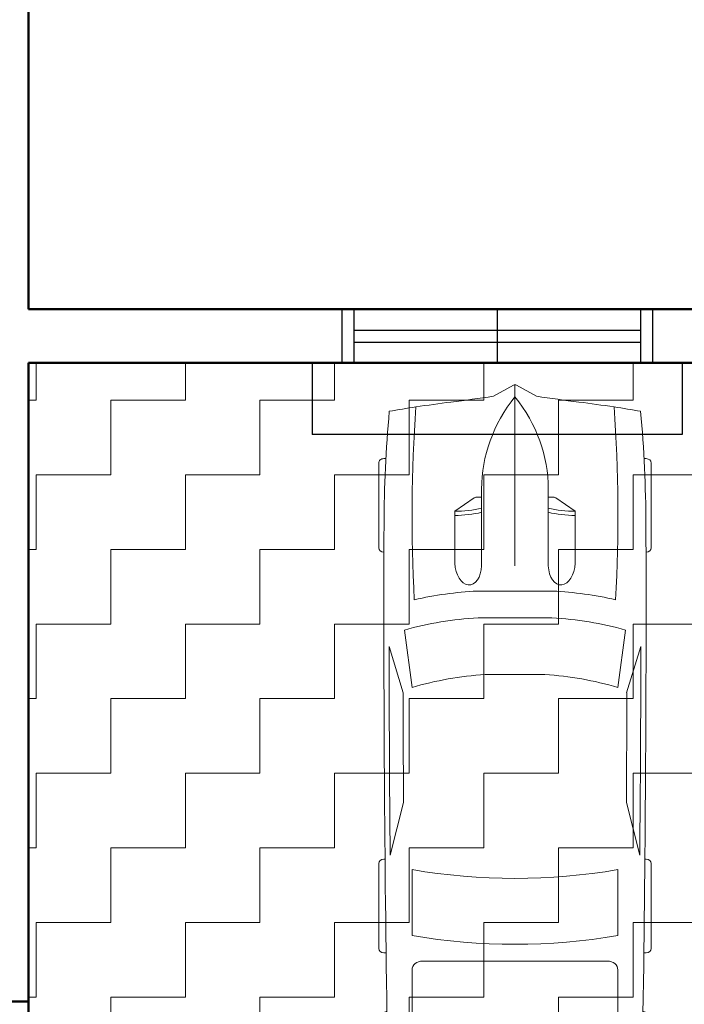
# Model space of a CAD drawing. Units: inches. Extents: x -105 to 1196, y -792 to 119.
# Tile 18 of 23: x 322 to 434, y -439 to -274. Entities that reach past the tile are written whole.
import ezdxf

# ---------------------------------------------------------------- set-up
doc = ezdxf.new("R2010")
doc.units = ezdxf.units.IN
doc.header["$MEASUREMENT"] = 0
for name, color, linetype, lineweight in [('A-EQPM', 8, 'Continuous', 18), ('A-FLOR-PATT', 252, 'Continuous', 13), ('A-GLAZ', 4, 'Continuous', 25), ('A-WALL', 3, 'Continuous', 50)]:
    doc.layers.add(name, color=color, linetype=linetype, lineweight=lineweight)

# ---------------------------------------------------------------- blocks, each defined once
blk = doc.blocks.new('*U19')
for p, q in [((21.1, 37.41), (21.1, 36.83)), ((46.55, 38.89), (22.35, 38.89)), ((47.8, 37.39), (47.8, 37.41)), ((135.45, 37.07), (135.45, 37.41)), ((136.7, 38.89), (160.9, 38.89)), ((162.15, 37.41), (162.15, 36.77)), ((87.99, 31.87), (74.76, 35.92)), ((134.31, 35.6), (119.29, 31.78)), ((70.03, 31.54), (86.41, 29.35)), ((186.47, -33.5), (186.47, 33.5)), ((188.4, -32.76), (188.4, 32.76)), ((138.42, 29.35), (157.25, 29.35)), ((186.47, 29.35), (167.01, 29.35)), ((164.52, 26.39), (164.52, -26.39)), ((32.27, 11.63), (36.13, 17.17)), ((36.13, 17.17), (50.94, 17.17)), ((29.77, 9.51), (51.68, 9.51)), ((32.12, 9.51), (32.12, 11.15)), ((58.92, -10.77), (58.92, 10.77)), ((66.55, -10.53), (66.55, 10.53)), ((82.74, 8.5), (82.74, -8.5)), ((186.47, -10.53), (186.47, 10.53)), ((3.27, 6.13), (0.1, 0.41)), ((0, 0), (51.68, 0)), ((0.1, -0.41), (3.27, -6.13)), ((29.77, -9.51), (51.68, -9.51)), ((32.12, -9.51), (32.12, -11.15)), ((32.27, -11.63), (36.13, -17.17)), ((36.13, -17.17), (50.94, -17.17)), ((86.41, -29.35), (70.03, -31.54)), ((157.25, -29.35), (138.42, -29.35)), ((167.01, -29.35), (186.47, -29.35)), ((87.99, -31.87), (74.76, -35.92)), ((134.31, -35.6), (119.29, -31.78)), ((21.1, -37.41), (21.1, -36.83)), ((46.55, -38.89), (22.35, -38.89)), ((47.8, -37.39), (47.8, -37.41)), ((135.45, -37.07), (135.45, -37.41)), ((136.7, -38.89), (160.9, -38.89)), ((162.15, -37.41), (162.15, -36.77))]:
    blk.add_line(p, q)
for centre, major_axis, ratio, start_param, end_param in [((41.19, -490.86), (0, 528.23), 0.842304, 0.00281, 0.075598), ((22.35, 37.41), (0, -1.48), 0.842304, 3.141593, 4.712389), ((64.48, -10555.62), (0, 10593.03), 0.842304, -0.013397, 0.002797), ((46.55, 37.41), (0, 1.48), 0.842304, -1.570796, 0), ((136.7, 37.41), (0, -1.48), 0.842304, 3.141593, 4.712389), ((160.9, 37.41), (0, 1.48), 0.842304, -1.570796, 0), ((180.63, 35.84), (0, 2.22), 0.842304, -0.013017, 1.249894), ((64.48, -10556.36), (0, 10595.31), 0.842304, -0.013397, -0.013017), ((183.98, 32.76), (0, -5.25), 0.842304, 1.570796, 3.128196), ((266.03, -27.52), (0, 313.31), 0.842304, 1.367076, 1.39176), ((64.48, -10555.62), (0, -10591.55), 0.842304, 3.133765, 3.140441), ((183.98, 33.5), (0, -2.96), 0.842304, 1.570796, 3.128196), ((135.29, 5.39), (0, 81.77), 0.842304, 1.245306, 1.50788), ((95.79, -3666.35), (0, -3698.24), 0.842304, 3.134049, 3.144098), ((259.18, -27.52), (0, -305.3), 0.842304, 4.528606, 4.561838), ((37.47, -593.96), (0, -623.33), 0.842304, 3.096046, 3.200911), ((134.4, 5.39), (0, -89.78), 0.842304, 4.449482, 4.652344), ((149.6, 2.8), (0, -79.58), 0.842304, 4.372215, 4.640744), ((17.08, 0), (0, 147.02), 0.842304, 4.511394, 4.913384), ((35.91, 0), (0, 147.02), 0.842304, 4.511394, 4.913384), ((167.01, 26.39), (0, 2.96), 0.842304, 0, 1.570796), ((-204.49, 52.4), (0, -250.96), 0.842304, 1.385369, 1.434372), ((13.04, 17.01), (0, 27.42), 0.842304, 4.435146, 4.718221), ((14.2, 17.01), (0, 27.42), 0.842304, 4.435146, 4.718221), ((50.79, 13.34), (6.34, -0.36), 0.603834, -1.395552, 1.581315), ((32.75, 11.15), (0, 0.74), 0.842304, 0.879714, 1.570796), ((29.77, -46.66), (0, 56.17), 0.842304, 0, 0.590319), ((0.62, 0), (0, -0.74), 0.842304, 4.131459, 5.293319), ((29.77, 46.66), (0, 56.17), 0.842304, 2.551274, 3.141593), ((-204.49, -52.4), (0, 250.96), 0.842304, -1.434372, -1.385369), ((32.75, -11.15), (0, -0.74), 0.842304, 4.712389, 5.403472), ((13.04, -17.01), (0, -27.42), 0.842304, 1.564964, 1.848039), ((14.2, -17.01), (0, -27.42), 0.842304, 1.564964, 1.848039), ((134.4, -5.39), (0, -89.78), 0.842304, -1.510751, -1.307889), ((135.29, -5.39), (0, -81.77), 0.842304, -1.50788, -1.245306), ((149.6, -2.8), (0, -79.58), 0.842304, -1.499151, -1.230623), ((259.18, 27.52), (0, 305.3), 0.842304, 1.721348, 1.754579), ((167.01, -26.39), (0, -2.96), 0.842304, 4.712389, 6.283185), ((266.03, 27.52), (0, 313.31), 0.842304, 1.749832, 1.774517), ((37.47, 593.96), (0, -623.33), 0.842304, -0.059319, 0.045547), ((95.79, 3666.35), (0, -3698.24), 0.842304, -0.002505, 0.007544), ((183.98, -33.5), (0, 2.96), 0.842304, 3.15499, 4.712389), ((183.98, -32.76), (0, -5.25), 0.842304, 0.013397, 1.570796), ((41.19, 490.86), (0, -528.23), 0.842304, -0.075598, -0.00281), ((64.48, 10555.62), (0, 10593.03), 0.842304, 3.138796, 3.15499), ((64.48, 10555.62), (0, -10591.55), 0.842304, 0.001152, 0.007828), ((180.63, -35.84), (0, -2.22), 0.842304, -1.249894, 0.013017), ((22.35, -37.41), (0, 1.48), 0.842304, 1.570796, 3.141593), ((46.55, -37.41), (0, -1.48), 0.842304, 0, 1.570796), ((136.7, -37.41), (0, -1.48), 0.842304, -1.570796, 0), ((160.9, -37.41), (0, 1.48), 0.842304, 3.141593, 4.712389), ((64.48, 10556.36), (0, 10595.31), 0.842304, 3.15461, 3.15499)]:
    blk.add_ellipse(centre, major_axis=major_axis, ratio=ratio, start_param=start_param, end_param=end_param)
at = {"extrusion": (0, 0, -1)}
blk.add_ellipse((50.79, -13.34), major_axis=(6.34, 0.36), ratio=0.603834, start_param=-1.395552, end_param=1.581315, dxfattribs=at)
blk = doc.blocks.new('WIN-1200')
at = {"ltscale": 2}
for p, q in [((12, 62), (0, 62)), ((0, 0), (0, 62)), ((12, 57), (12, 62)), ((12, 5), (12, 0)), ((12, 0), (0, 0))]:
    blk.add_line(p, q, dxfattribs=at)
for p, q in [((21, 57), (12, 57)), ((21, 5), (12, 5))]:
    blk.add_line(p, q)

msp = doc.modelspace()

# ---------------------------------------------------------------- hatches: boundary and pattern name
at = {"layer": 'A-FLOR-PATT'}
h = msp.add_hatch(dxfattribs=at)
h.set_pattern_fill('ZIGZAG', color=256, scale=100)
h.set_pattern_definition([(0, (0, 0), (12.5, 12.5), [12.5, -12.5]), (90, (12.5, 0), (-12.5, 12.5), [12.5, -12.5])])
h.paths.add_polyline_path([(489.74, -331.23), (323.74, -331.23), (323.74, -508.23), (489.74, -508.23)])
h.paths.add_polyline_path([(383.72, -476.81), (434.09, -476.81), (434.09, -454.42), (383.72, -454.42)], flags=24)

# ---------------------------------------------------------------- linework, layer by layer
at = {"layer": 'A-GLAZ'}
for p, q in [((378.24, -322.23), (378.24, -331.23)), ((402.24, -322.23), (402.24, -331.23)), ((426.24, -322.23), (426.24, -331.23)), ((378.24, -325.73), (426.24, -325.73)), ((378.24, -327.73), (426.24, -327.73))]:
    msp.add_line(p, q, dxfattribs=at)
at = {"layer": 'A-WALL'}
for p, q in [((323.74, -267.77), (323.74, -322.23)), ((480.74, -322.23), (323.74, -322.23)), ((489.74, -331.23), (323.74, -331.23)), ((323.74, -331.23), (323.74, -508.23)), ((188.8, -438.23), (323.74, -438.23))]:
    msp.add_line(p, q, dxfattribs=at)

# ---------------------------------------------------------------- block references
at = {"layer": 'A-EQPM', "xscale": 0.5869636799172785, "yscale": 0.5869636799172785, "zscale": 0.5869636799172785, "rotation": 270}
msp.add_blockref('*U19', (405.22, -334.89), dxfattribs=at)
at = {"layer": 'A-GLAZ', "rotation": 90.00000000000011}
msp.add_blockref('WIN-1200', (433.24, -343.23), dxfattribs=at)

doc.saveas('drawing.dxf')
